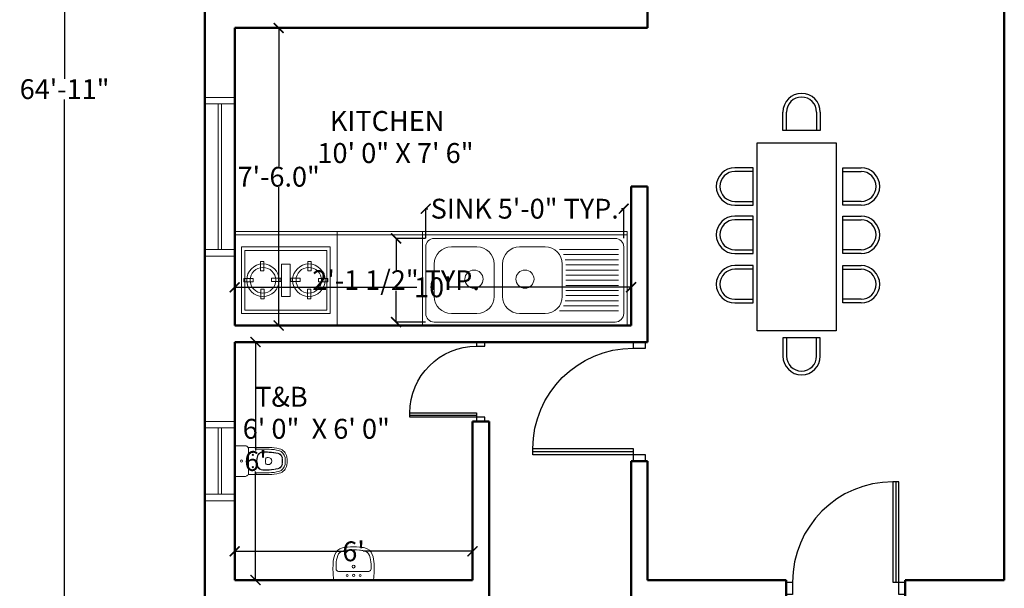
# Model space of a CAD drawing. Units: inches. Extents: x 147 to 1638, y 107 to 941.
# Tile 13 of 17: x 1062 to 1360, y 398 to 570. Entities that reach past the tile are written whole.
import ezdxf

# ---------------------------------------------------------------- set-up
doc = ezdxf.new("R2010")
doc.units = ezdxf.units.IN
doc.header["$MEASUREMENT"] = 0
for name, color, linetype, lineweight in [('A-ANNO-DIMS', 2, 'Continuous', 15), ('A-AREA-IDEN', 7, 'Continuous', 18), ('A-Door', 150, 'Continuous', 25), ('A-EQPM', 8, 'Continuous', 18), ('A-FLOR-CASE', 9, 'Continuous', 20), ('A-FLOR-FIXT', 9, 'Continuous', 18), ('furniture', 50, 'Continuous', 18), ('walls', 7, 'Continuous', 50), ('windows', 3, 'Continuous', 20)]:
    doc.layers.add(name, color=color, linetype=linetype, lineweight=lineweight)
for name, color, linetype in [('A-Glaz', 92, 'Continuous'), ('NT', 1, 'Continuous'), ('家', 40, 'Continuous')]:
    doc.layers.add(name, color=color, linetype=linetype)
doc.styles.get("Standard").update_dxf_attribs({"font": 'arial.ttf'})
doc.dimstyles.get("Standard").update_dxf_attribs({"dimtxt": 6, "dimasz": 3, "dimexe": 0.18, "dimexo": 0.0625, "dimgap": 0.09, "dimtad": 0, "dimtih": 1, "dimtoh": 1, "dimdec": 1, "dimzin": 0, "dimdsep": 46, "dimlunit": 3, "dimtxsty": 'Standard', "dimblk": 'ARCHTICK', "dimcen": 0.09, "dimadec": 0, "dimazin": 0, "dimtfac": 1, "dimtdec": 1, "dimtofl": 0, "dimtmove": 0, "dimatfit": 3, "dimfxl": 1, "dimtolj": 1, "dimtzin": 0, "dimarcsym": 0})

# ---------------------------------------------------------------- blocks, each defined once
blk = doc.blocks.new('A$C087A3AA9')
at = {"layer": 'A-Door'}
for points in [[(852.6, 94.7), (852.6, 852.6), (805.3, 852.6), (805.3, 94.7)], [(47.4, 94.7), (47.4, 0), (0, 0), (0, 94.7)], [(900, 94.7), (900, 0), (852.6, 0), (852.6, 94.7)]]:
    blk.add_lwpolyline(points, close=True, dxfattribs=at)
at = {"layer": 'A-Glaz'}
blk.add_line((828.9, 852.6), (828.9, 94.7), dxfattribs=at)
at = {"layer": 'NT'}
blk.add_arc((805.3, 94.7), 757.9, 90, 180, dxfattribs=at)
blk = doc.blocks.new('_ArchTick')
at = {"color": 0, "linetype": 'ByBlock', "const_width": 0.15}
blk.add_lwpolyline([(-0.5, -0.5), (0.5, 0.5)], dxfattribs=at)
blk = doc.blocks.new('*D59')
at = {"layer": 'A-ANNO-DIMS', "color": 0, "lineweight": -2, "transparency": 16777216}
for p, q in [((1133.05, 567.72), (1140.27, 567.72)), ((1140.09, 567.72), (1140.09, 525.87)), ((1140.09, 477.72), (1140.09, 519.56)), ((1133.05, 477.72), (1140.27, 477.72))]:
    blk.add_line(p, q, dxfattribs=at)
at = {"layer": 'Defpoints', "color": 0, "lineweight": -2, "transparency": 16777216}
for p in [(1132.98, 567.72), (1132.98, 477.72), (1140.09, 477.72)]:
    blk.add_point(p, dxfattribs=at)
at = {"layer": 'A-ANNO-DIMS', "color": 0, "lineweight": -2, "transparency": 16777216, "xscale": 3, "yscale": 3, "zscale": 3}
for p, rotation in [((1140.09, 567.72), 90), ((1140.09, 477.72), 270)]:
    blk.add_blockref('_ArchTick', p, dxfattribs=dict(at, rotation=rotation))
at = {"layer": 'A-ANNO-DIMS', "color": 0, "transparency": 16777216, "insert": (1140.09, 522.72), "char_height": 6, "attachment_point": 5}
blk.add_mtext('\\A1;7\'-6.0"', dxfattribs=at)
blk = doc.blocks.new('*D60')
at = {"layer": 'A-ANNO-DIMS', "color": 0, "lineweight": -2, "transparency": 16777216}
for p, q in [((1126.77, 486.05), (1126.77, 489.45)), ((1126.77, 489.27), (1181.87, 489.27)), ((1246.77, 489.27), (1191.67, 489.27)), ((1246.77, 486.05), (1246.77, 489.45))]:
    blk.add_line(p, q, dxfattribs=at)
at = {"layer": 'Defpoints', "color": 0, "lineweight": -2, "transparency": 16777216}
for p in [(1246.77, 489.27), (1126.77, 485.98), (1246.77, 485.98)]:
    blk.add_point(p, dxfattribs=at)
at = {"layer": 'A-ANNO-DIMS', "color": 0, "lineweight": -2, "transparency": 16777216, "xscale": 3, "yscale": 3, "zscale": 3, "rotation": 180}
blk.add_blockref('_ArchTick', (1126.77, 489.27), dxfattribs=at)
at = {"layer": 'A-ANNO-DIMS', "color": 0, "lineweight": -2, "transparency": 16777216, "xscale": 3, "yscale": 3, "zscale": 3}
blk.add_blockref('_ArchTick', (1246.77, 489.27), dxfattribs=at)
at = {"layer": 'A-ANNO-DIMS', "color": 0, "transparency": 16777216, "insert": (1186.77, 489.27), "char_height": 6, "attachment_point": 5}
blk.add_mtext("\\A1;10'", dxfattribs=at)
blk = doc.blocks.new('*D61')
at = {"layer": 'A-ANNO-DIMS', "color": 0, "lineweight": -2, "transparency": 16777216}
for p, q in [((1131.42, 472.72), (1133.26, 472.72)), ((1133.08, 472.72), (1133.08, 439.87)), ((1133.08, 400.72), (1133.08, 433.56)), ((1131.42, 400.72), (1133.26, 400.72))]:
    blk.add_line(p, q, dxfattribs=at)
at = {"layer": 'Defpoints', "color": 0, "lineweight": -2, "transparency": 16777216}
for p in [(1131.36, 472.72), (1131.36, 400.72), (1133.08, 400.72)]:
    blk.add_point(p, dxfattribs=at)
at = {"layer": 'A-ANNO-DIMS', "color": 0, "lineweight": -2, "transparency": 16777216, "xscale": 3, "yscale": 3, "zscale": 3}
for p, rotation in [((1133.08, 472.72), 90), ((1133.08, 400.72), 270)]:
    blk.add_blockref('_ArchTick', p, dxfattribs=dict(at, rotation=rotation))
at = {"layer": 'A-ANNO-DIMS', "color": 0, "transparency": 16777216, "insert": (1133.08, 436.72), "char_height": 6, "attachment_point": 5}
blk.add_mtext("\\A1;6'", dxfattribs=at)
blk = doc.blocks.new('*D62')
at = {"layer": 'A-ANNO-DIMS', "color": 0, "lineweight": -2, "transparency": 16777216}
for p, q in [((1126.77, 409.46), (1126.77, 409.58)), ((1126.77, 409.4), (1159.9, 409.4)), ((1198.77, 409.4), (1165.63, 409.4)), ((1198.77, 409.46), (1198.77, 409.58))]:
    blk.add_line(p, q, dxfattribs=at)
at = {"layer": 'Defpoints', "color": 0, "lineweight": -2, "transparency": 16777216}
for p in [(1126.77, 409.4), (1198.77, 409.4), (1198.77, 409.4)]:
    blk.add_point(p, dxfattribs=at)
at = {"layer": 'A-ANNO-DIMS', "color": 0, "lineweight": -2, "transparency": 16777216, "xscale": 3, "yscale": 3, "zscale": 3, "rotation": 180}
blk.add_blockref('_ArchTick', (1126.77, 409.4), dxfattribs=at)
at = {"layer": 'A-ANNO-DIMS', "color": 0, "lineweight": -2, "transparency": 16777216, "xscale": 3, "yscale": 3, "zscale": 3}
blk.add_blockref('_ArchTick', (1198.77, 409.4), dxfattribs=at)
at = {"layer": 'A-ANNO-DIMS', "color": 0, "transparency": 16777216, "insert": (1162.77, 409.4), "char_height": 6, "attachment_point": 5}
blk.add_mtext("\\A1;6'", dxfattribs=at)
blk = doc.blocks.new('2SAINDA')
at = {"color": 0, "linetype": 'ByBlock'}
for p, q in [((0, 0.188), (0, -0.188)), ((0.018, 0.2), (0.141, 0.2)), ((0.157, 0.192), (0.162, 0.188)), ((0.18, -0.164), (0.18, 0.164)), ((0.279, 0.159), (0.261, 0.176)), ((0.437, 0.047), (0.424, 0.047)), ((0.437, -0.047), (0.424, -0.047)), ((0.018, -0.2), (0.141, -0.2)), ((0.157, -0.192), (0.162, -0.188)), ((0.279, -0.159), (0.261, -0.176))]:
    blk.add_line(p, q, dxfattribs=at)
for centre, radius in [((0.09, 0), 0.0135), ((0.09, 0), 0.0135), ((0.236, 0.08), 0.0075), ((0.236, -0.08), 0.0075)]:
    blk.add_circle(centre, radius, dxfattribs=at)
for centre, radius, start, end in [((0.018, 0.18), 0.02, 90, 155.6901), ((0.141, 0.181), 0.019, 34.9372, 90), ((0.155, 0.164), 0.025, 23.3776, 73.7848), ((0.383, -5.322), 5.5, 89.2905, 92.1362), ((0.155, 0.164), 0.025, 360, 23.3776), ((0.293, 0.173), 0.02, 225, 270.9364), ((0.383, -5.322), 5.476, 89.2905, 90.9364), ((0.444, -0.373), 0.55, 75.4605, 89.2905), ((0.444, -0.373), 0.526, 75.4605, 89.2905), ((0.549, 0.03), 0.11, 8.8162, 75.4605), ((0.549, 0.03), 0.134, 8.8162, 75.4605), ((0.485, 0), 0.2, 160.016, 199.984), ((0.485, 0), 0.196, 160.016, 199.984), ((0.368, 0.043), 0.075, 90.1648, 160.016), ((0.368, 0.043), 0.071, 90.1648, 160.016), ((0.383, -5.322), 5.44, 89.2905, 90.1648), ((0.383, -5.322), 5.436, 89.2905, 90.1648), ((0.582, 0), 0.18, 170.2849, 189.7151), ((0.424, 0.027), 0.02, 90, 170.2849), ((0.437, 0), 0.047, 0, 90), ((0.437, 0), 0.047, 270, 0), ((0.444, -0.373), 0.49, 75.4605, 89.2905), ((0.444, -0.373), 0.486, 75.4605, 89.2905), ((0.549, 0.03), 0.07, 8.8162, 75.4605), ((0.549, 0.03), 0.074, 8.8162, 75.4605), ((0.355, 0), 0.266, 351.1838, 8.8162), ((0.355, 0), 0.27, 351.1838, 8.8162), ((0.355, 0), 0.306, 351.1838, 8.8162), ((0.355, 0), 0.33, 351.1838, 8.8162), ((0.368, -0.043), 0.075, 199.984, 269.8352), ((0.368, -0.043), 0.071, 199.984, 269.8352), ((0.383, 5.322), 5.436, 269.8352, 270.7095), ((0.383, 5.322), 5.44, 269.8352, 270.7095), ((0.424, -0.027), 0.02, 189.7151, 270), ((0.444, 0.373), 0.486, 270.7095, 284.5395), ((0.444, 0.373), 0.49, 270.7095, 284.5395), ((0.549, -0.03), 0.07, 284.5395, 351.1838), ((0.549, -0.03), 0.074, 284.5395, 351.1838), ((0.549, -0.03), 0.11, 284.5395, 351.1838), ((0.549, -0.03), 0.134, 284.5395, 351.1838), ((0.018, -0.18), 0.02, 204.3099, 270), ((0.141, -0.181), 0.019, 270, 325.0628), ((0.155, -0.164), 0.025, 286.2152, 336.6224), ((0.155, -0.164), 0.025, 336.6224, 0), ((0.383, 5.322), 5.5, 267.8638, 270.7095), ((0.293, -0.173), 0.02, 89.0636, 135), ((0.383, 5.322), 5.476, 269.0636, 270.7095), ((0.444, 0.373), 0.526, 270.7095, 284.5395), ((0.444, 0.373), 0.55, 270.7095, 284.5395)]:
    blk.add_arc(centre, radius, start, end, dxfattribs=at)
blk = doc.blocks.new('2SALADA2')
at = {"color": 0}
for p, q in [((-0.296, 0), (0.296, 0)), ((0.207, -0.13), (-0.207, -0.13))]:
    blk.add_line(p, q, dxfattribs=at)
for centre, radius in [((-0.1, -0.07), 0.015), ((0, -0.07), 0.0175), ((0.1, -0.07), 0.015), ((0, -0.205), 0.023)]:
    blk.add_circle(centre, radius, dxfattribs=at)
for centre, radius, start, end in [((-0.296, -0.01), 0.01, 90, 173.6262), ((0.296, -0.01), 0.01, 6.3738, 90), ((1.185, -0.175), 1.5, 173.6262, 182.693), ((-0.227, -0.171), 0.04, 95.5937, 179.6995), ((-0.207, -0.38), 0.25, 90, 95.5937), ((0.207, -0.38), 0.25, 84.4063, 90), ((0.227, -0.171), 0.04, 0.3005, 84.4063), ((-1.185, -0.175), 1.5, 357.307, 6.3738), ((0.186, -0.222), 0.5, 182.693, 199.3406), ((1.186, -0.221), 1.454, 178.0234, 180.898), ((0.186, -0.222), 0.454, 182.693, 199.3406), ((-0.186, -0.222), 0.454, 340.6594, 357.307), ((-1.186, -0.221), 1.454, 359.102, 1.9766), ((-0.186, -0.222), 0.5, 340.6594, 357.307), ((-0.135, -0.335), 0.16, 199.3406, 257.4429), ((-0.135, -0.335), 0.114, 199.3406, 257.4429), ((-0.061, -0.003), 0.454, 257.4429, 266.4982), ((0.061, -0.003), 0.454, 273.5018, 282.5571), ((0.135, -0.335), 0.114, 282.5571, 340.6594), ((0.135, -0.335), 0.16, 282.5571, 340.6594), ((-0.061, -0.003), 0.5, 257.4429, 266.4982), ((0, 0.995), 1.5, 266.4982, 273.5018), ((0, 0.995), 1.454, 266.4982, 273.5018), ((0.061, -0.003), 0.5, 273.5018, 282.5571)]:
    blk.add_arc(centre, radius, start, end, dxfattribs=at)
blk = doc.blocks.new('A$C45A766E2')
at = {"layer": '家'}
for p, q in [((0.363, 1.317), (0.363, 1.078)), ((0.412, 1.317), (0.412, 1.078)), ((0.801, 1.078), (0.801, 1.317)), ((0.849, 1.078), (0.849, 1.317)), ((1.006, 1.317), (1.006, 1.078)), ((1.054, 1.317), (1.054, 1.078)), ((1.443, 1.078), (1.443, 1.317)), ((1.492, 1.078), (1.492, 1.317)), ((1.634, 1.317), (1.634, 1.078)), ((1.683, 1.317), (1.683, 1.078)), ((2.072, 1.078), (2.072, 1.317)), ((2.12, 1.078), (2.12, 1.317)), ((0, 1.028), (2.445, 1.028)), ((0, 0), (0, 1.028)), ((0.363, 1.078), (0.849, 1.078)), ((0.363, 1.078), (0.849, 1.078)), ((1.006, 1.078), (1.492, 1.078)), ((1.006, 1.078), (1.492, 1.078)), ((1.634, 1.078), (2.12, 1.078)), ((1.634, 1.078), (2.12, 1.078)), ((2.445, 1.028), (2.445, 0)), ((-0.088, 0.693), (-0.327, 0.693)), ((-0.088, 0.644), (-0.327, 0.644)), ((-0.088, 0.207), (-0.088, 0.693)), ((-0.088, 0.207), (-0.088, 0.693)), ((2.604, 0.693), (2.843, 0.693)), ((2.604, 0.207), (2.604, 0.693)), ((2.604, 0.207), (2.604, 0.693)), ((2.604, 0.644), (2.843, 0.644)), ((-0.327, 0.255), (-0.088, 0.255)), ((-0.327, 0.207), (-0.088, 0.207)), ((2.843, 0.255), (2.604, 0.255)), ((2.843, 0.207), (2.604, 0.207)), ((2.445, 0), (0, 0)), ((0.363, -0.085), (0.849, -0.085)), ((0.363, -0.085), (0.849, -0.085)), ((0.363, -0.324), (0.363, -0.085)), ((0.412, -0.324), (0.412, -0.085)), ((0.801, -0.085), (0.801, -0.324)), ((0.849, -0.085), (0.849, -0.324)), ((1.006, -0.324), (1.006, -0.085)), ((1.006, -0.085), (1.492, -0.085)), ((1.006, -0.085), (1.492, -0.085)), ((1.054, -0.324), (1.054, -0.085)), ((1.443, -0.085), (1.443, -0.324)), ((1.492, -0.085), (1.492, -0.324)), ((1.634, -0.085), (2.12, -0.085)), ((1.634, -0.085), (2.12, -0.085)), ((1.634, -0.324), (1.634, -0.085)), ((1.683, -0.324), (1.683, -0.085)), ((2.072, -0.085), (2.072, -0.324)), ((2.12, -0.085), (2.12, -0.324))]:
    blk.add_line(p, q, dxfattribs=at)
for centre, radius, start, end in [((0.606, 1.317), 0.243, 0, 180), ((1.249, 1.317), 0.243, 0, 180), ((1.877, 1.317), 0.243, 0, 180), ((0.606, 1.317), 0.195, 0, 180), ((1.249, 1.317), 0.195, 0, 180), ((1.877, 1.317), 0.195, 0, 180), ((-0.327, 0.45), 0.243, 90, 270), ((-0.327, 0.45), 0.195, 90, 270), ((2.843, 0.45), 0.243, 270, 90), ((2.843, 0.45), 0.195, 270, 90), ((0.606, -0.324), 0.243, 180, 0), ((0.606, -0.324), 0.195, 180, 0), ((1.249, -0.324), 0.243, 180, 0), ((1.249, -0.324), 0.195, 180, 0), ((1.877, -0.324), 0.243, 180, 0), ((1.877, -0.324), 0.195, 180, 0)]:
    blk.add_arc(centre, radius, start, end, dxfattribs=at)
blk = doc.blocks.new('WIN-48IN')
for p, q in [((9, 48), (0, 48)), ((0, 48), (0, 0)), ((9, 0), (9, 48)), ((9, 46), (0, 46)), ((4, 2), (4, 46)), ((5, 2), (5, 46)), ((0, 2), (9, 2)), ((0, 0), (9, 0))]:
    blk.add_line(p, q)
blk = doc.blocks.new('WIN-24IN')
for p, q in [((9, 24), (0, 24)), ((0, 24), (0, 0)), ((9, 0), (9, 24)), ((9, 22), (0, 22)), ((4, 2), (4, 22)), ((5, 2), (5, 22)), ((0, 2), (9, 2)), ((0, 0), (9, 0))]:
    blk.add_line(p, q)
blk = doc.blocks.new('CABINET-KITCHEN-RUN')
for p, q in [((0, 28.41), (118.8, 28.41)), ((0, 0), (0, 28.41)), ((0, 27.38), (118.8, 27.38)), ((30.99, 0), (30.99, 28.41)), ((56.82, 0), (56.82, 28.41)), ((118.8, 28.41), (118.8, 0)), ((118.8, 0), (0, 0))]:
    blk.add_line(p, q)
blk = doc.blocks.new('COOKTOP-2-BURNER')
for p, q in [((0, 0), (0, 20.15)), ((0, 20.15), (26.86, 20.15)), ((1.03, 1.03), (1.03, 19.11)), ((1.03, 19.11), (25.83, 19.11)), ((25.83, 1.03), (25.83, 19.11)), ((26.86, 0), (26.86, 20.15)), ((5.75, 15.75), (5.75, 12.91)), ((5.75, 15.75), (6.79, 15.75)), ((6.79, 15.75), (6.79, 12.91)), ((12.14, 14.98), (14.72, 14.98)), ((12.14, 14.98), (12.14, 5.17)), ((14.72, 14.98), (14.72, 5.17)), ((21.11, 15.75), (20.07, 15.75)), ((20.07, 15.75), (20.07, 12.91)), ((21.11, 15.75), (21.11, 12.91)), ((5.75, 12.91), (6.79, 12.91)), ((21.11, 12.91), (20.07, 12.91)), ((0.69, 9.55), (0.69, 10.59)), ((0.69, 10.59), (3.53, 10.59)), ((0.69, 9.55), (3.53, 9.55)), ((3.53, 9.55), (3.53, 10.59)), ((11.95, 10.69), (9.11, 10.69)), ((9.11, 10.69), (9.11, 9.66)), ((11.95, 9.66), (9.11, 9.66)), ((11.95, 10.69), (11.95, 9.66)), ((14.91, 10.69), (17.75, 10.69)), ((14.91, 10.69), (14.91, 9.66)), ((14.91, 9.66), (17.75, 9.66)), ((17.75, 10.69), (17.75, 9.66)), ((23.33, 9.55), (23.33, 10.59)), ((26.17, 10.59), (23.33, 10.59)), ((26.17, 9.55), (23.33, 9.55)), ((26.17, 9.55), (26.17, 10.59)), ((5.86, 4.49), (5.86, 7.33)), ((6.89, 7.33), (5.86, 7.33)), ((6.89, 4.49), (6.89, 7.33)), ((19.97, 4.49), (19.97, 7.33)), ((19.97, 7.33), (21, 7.33)), ((21, 4.49), (21, 7.33)), ((6.89, 4.49), (5.86, 4.49)), ((12.14, 5.17), (14.72, 5.17)), ((19.97, 4.49), (21, 4.49)), ((0, 0), (26.86, 0)), ((1.03, 1.03), (25.83, 1.03))]:
    blk.add_line(p, q)
for centre, radius in [((6.48, 10.08), 4.91), ((20.38, 10.08), 4.91), ((6.48, 10.08), 3.87), ((20.38, 10.08), 3.87)]:
    blk.add_circle(centre, radius)
blk = doc.blocks.new('SINK-DOUBLE-DRAINBOARD')
for p, q in [((57.34, 25.31), (2.58, 25.31)), ((0, 22.73), (0, 2.58)), ((15.5, 22.73), (7.75, 22.73)), ((36.16, 22.73), (28.41, 22.73)), ((40.53, 21.95), (58.37, 21.95)), ((59.92, 2.58), (59.92, 22.73)), ((41.67, 20.4), (58.37, 20.4)), ((42.22, 18.85), (58.37, 18.85)), ((2.58, 17.56), (2.58, 7.75)), ((20.66, 17.56), (20.66, 7.75)), ((23.24, 17.56), (23.24, 7.75)), ((41.32, 17.56), (41.32, 7.75)), ((42.36, 17.3), (58.37, 17.3)), ((42.36, 15.75), (58.37, 15.75)), ((42.36, 14.2), (58.37, 14.2)), ((42.36, 12.66), (58.37, 12.66)), ((42.36, 11.11), (58.37, 11.11)), ((42.36, 9.56), (58.37, 9.56)), ((42.22, 6.46), (58.37, 6.46)), ((42.36, 8.01), (58.37, 8.01)), ((40.53, 3.36), (58.37, 3.36)), ((41.67, 4.91), (58.37, 4.91)), ((2.58, 0), (57.34, 0)), ((7.75, 2.58), (15.5, 2.58)), ((28.41, 2.58), (36.16, 2.58))]:
    blk.add_line(p, q)
for centre in [(14.61, 13), (30.02, 13)]:
    blk.add_circle(centre, 2.75)
for centre, radius, start, end in [((2.58, 22.73), 2.58, 90, 180), ((57.34, 22.73), 2.58, 0, 90), ((7.75, 17.56), 5.17, 90, 180), ((15.5, 17.56), 5.17, 0, 90), ((28.41, 17.56), 5.17, 90, 180), ((36.16, 17.56), 5.17, 0, 90), ((7.75, 7.75), 5.17, 180, 270), ((15.5, 7.75), 5.17, 270, 0), ((28.41, 7.75), 5.17, 180, 270), ((36.16, 7.75), 5.17, 270, 0), ((2.58, 2.58), 2.58, 180, 270), ((57.34, 2.58), 2.58, 270, 0)]:
    blk.add_arc(centre, radius, start, end)
blk = doc.blocks.new('*D126')
at = {"layer": 'A-ANNO-DIMS', "color": 0, "lineweight": -2, "transparency": 16777216}
for p, q in [((1184.62, 504.12), (1184.62, 513.23)), ((1184.62, 513.05), (1185.27, 513.05)), ((1244.54, 513.05), (1243.89, 513.05)), ((1244.54, 504.12), (1244.54, 513.23))]:
    blk.add_line(p, q, dxfattribs=at)
at = {"layer": 'Defpoints', "color": 0, "lineweight": -2, "transparency": 16777216}
for p in [(1244.54, 513.05), (1184.62, 504.06), (1244.54, 504.06)]:
    blk.add_point(p, dxfattribs=at)
at = {"layer": 'A-ANNO-DIMS', "color": 0, "lineweight": -2, "transparency": 16777216, "xscale": 3, "yscale": 3, "zscale": 3, "rotation": 180}
blk.add_blockref('_ArchTick', (1184.62, 513.05), dxfattribs=at)
at = {"layer": 'A-ANNO-DIMS', "color": 0, "lineweight": -2, "transparency": 16777216, "xscale": 3, "yscale": 3, "zscale": 3}
blk.add_blockref('_ArchTick', (1244.54, 513.05), dxfattribs=at)
at = {"layer": 'A-ANNO-DIMS', "color": 0, "transparency": 16777216, "insert": (1214.58, 513.05), "char_height": 6, "attachment_point": 5}
blk.add_mtext('\\A1;SINK 5\'-0" TYP.', dxfattribs=at)
blk = doc.blocks.new('*D127')
at = {"layer": 'A-ANNO-DIMS', "color": 0, "lineweight": -2, "transparency": 16777216}
for p, q in [((1184.56, 504.06), (1175.45, 504.06)), ((1175.63, 504.06), (1175.63, 494.6)), ((1175.63, 478.75), (1175.63, 488.21)), ((1184.56, 478.75), (1175.45, 478.75))]:
    blk.add_line(p, q, dxfattribs=at)
at = {"layer": 'Defpoints', "color": 0, "lineweight": -2, "transparency": 16777216}
for p in [(1175.63, 504.06), (1184.62, 504.06), (1184.62, 478.75)]:
    blk.add_point(p, dxfattribs=at)
at = {"layer": 'A-ANNO-DIMS', "color": 0, "lineweight": -2, "transparency": 16777216, "xscale": 3, "yscale": 3, "zscale": 3}
for p, rotation in [((1175.63, 504.06), 90), ((1175.63, 478.75), 270)]:
    blk.add_blockref('_ArchTick', p, dxfattribs=dict(at, rotation=rotation))
at = {"layer": 'A-ANNO-DIMS', "color": 0, "transparency": 16777216, "insert": (1175.63, 491.41), "char_height": 6, "attachment_point": 5}
blk.add_mtext('\\A1;2\'-1 1/2" TYP.', dxfattribs=at)
blk = doc.blocks.new('*D135')
at = {"layer": 'A-ANNO-DIMS', "color": 0, "lineweight": -2, "transparency": 16777216}
for p, q in [((1176.71, 938.72), (1075.09, 938.72)), ((1075.27, 938.72), (1075.27, 552.37)), ((1075.27, 159.72), (1075.27, 546.06)), ((1117.71, 159.72), (1075.09, 159.72))]:
    blk.add_line(p, q, dxfattribs=at)
at = {"layer": 'Defpoints', "color": 0, "lineweight": -2, "transparency": 16777216}
for p in [(1075.27, 938.72), (1176.77, 938.72), (1117.77, 159.72)]:
    blk.add_point(p, dxfattribs=at)
at = {"layer": 'A-ANNO-DIMS', "color": 0, "lineweight": -2, "transparency": 16777216, "xscale": 3, "yscale": 3, "zscale": 3}
for p, rotation in [((1075.27, 938.72), 90), ((1075.27, 159.72), 270)]:
    blk.add_blockref('_ArchTick', p, dxfattribs=dict(at, rotation=rotation))
at = {"layer": 'A-ANNO-DIMS', "color": 0, "transparency": 16777216, "insert": (1075.27, 549.22), "char_height": 6, "attachment_point": 5}
blk.add_mtext('\\A1;64\'-11"', dxfattribs=at)

msp = doc.modelspace()

# ---------------------------------------------------------------- linework, layer by layer
at = {"layer": 'walls'}
for p, q in [((1117.77, 909.72), (1117.77, 201.72)), ((1359.77, 722.72), (1359.77, 400.72)), ((1251.77, 572.72), (1251.77, 567.72)), ((1126.77, 567.72), (1126.77, 477.72)), ((1126.77, 567.72), (1246.77, 567.72)), ((1246.77, 567.72), (1251.77, 567.72)), ((1246.77, 519.72), (1246.77, 477.72)), ((1246.77, 519.72), (1251.77, 519.72)), ((1251.77, 519.72), (1251.77, 472.72)), ((1126.77, 477.72), (1246.77, 477.72)), ((1126.77, 472.72), (1126.77, 400.72)), ((1126.77, 472.72), (1198.77, 472.72)), ((1203.77, 472.72), (1198.77, 472.72)), ((1203.77, 472.72), (1246.77, 472.72)), ((1246.77, 472.72), (1251.77, 472.72)), ((1198.77, 448.72), (1198.77, 400.72)), ((1203.77, 448.72), (1198.77, 448.72)), ((1203.77, 448.72), (1203.77, 395.72)), ((1246.77, 436.72), (1246.77, 210.72)), ((1246.77, 436.72), (1251.77, 436.72)), ((1251.77, 436.72), (1251.77, 400.72)), ((1126.77, 400.72), (1198.77, 400.72)), ((1251.77, 400.72), (1281.77, 400.72)), ((1281.77, 400.72), (1293.77, 400.72)), ((1293.77, 400.72), (1293.77, 395.72)), ((1329.77, 400.72), (1359.77, 400.72)), ((1329.77, 400.72), (1329.77, 395.72))]:
    msp.add_line(p, q, dxfattribs=at)

# ---------------------------------------------------------------- block references
at = {"layer": 'A-Door', "rotation": 90}
for p, xscale, yscale, zscale in [((1202.53, 472.72), -0.0266666667542921, 0.0266666667542921, 0.0266666667542921), ((1251.16, 472.72), -0.0400000000000001, 0.0400000000000001, 0.0400000000000001)]:
    msp.add_blockref('A$C087A3AA9', p, dxfattribs=dict(at, xscale=xscale, yscale=yscale, zscale=zscale))
at = {"layer": 'A-Door', "xscale": 0.0400000000000001, "yscale": 0.0400000000000001, "zscale": 0.0400000000000001}
msp.add_blockref('A$C087A3AA9', (1293.77, 396.32), dxfattribs=at)
at = {"layer": 'A-EQPM'}
msp.add_blockref('COOKTOP-2-BURNER', (1128.83, 481.33), dxfattribs=at)
at = {"layer": 'A-FLOR-CASE'}
msp.add_blockref('CABINET-KITCHEN-RUN', (1126.77, 477.72), dxfattribs=at)
at = {"layer": 'A-FLOR-FIXT'}
msp.add_blockref('SINK-DOUBLE-DRAINBOARD', (1184.62, 478.75), dxfattribs=at)
at = {"layer": 'A-FLOR-FIXT', "xscale": 23.19012112898009, "yscale": 23.19012112898009, "zscale": 23.19012112898009}
msp.add_blockref('2SAINDA', (1126.77, 436.72), dxfattribs=at)
at = {"layer": 'A-FLOR-FIXT', "xscale": 19.81841434140962, "yscale": 19.81841434140962, "zscale": 19.81841434140962, "rotation": 180}
msp.add_blockref('2SALADA2', (1162.77, 400.72), dxfattribs=at)
at = {"layer": 'furniture', "xscale": 23.28367368005433, "yscale": 23.28367368005433, "zscale": 23.28367368005433, "rotation": 90}
msp.add_blockref('A$C45A766E2', (1308.87, 476.07), dxfattribs=at)
at = {"layer": 'windows'}
for name, p in [('WIN-48IN', (1117.77, 498.72)), ('WIN-24IN', (1117.77, 424.72))]:
    msp.add_blockref(name, p, dxfattribs=at)

# ---------------------------------------------------------------- texts
at = {"layer": 'A-AREA-IDEN'}
for s, height, p in [('KITCHEN ', 6.031, (1155.57, 536.56)), ('  10\' 0" X 7\' 6"', 6.0306, (1148.12, 526.87)), ('T&B', 6.031, (1132.95, 453.14)), ('  6\' 0"  X 6\' 0"', 6.0306, (1125.51, 443.45))]:
    msp.add_text(s, height=height, dxfattribs=at).set_placement(p)

# ---------------------------------------------------------------- dimensions: what is measured, and where the dimension line sits
at = {"layer": 'A-ANNO-DIMS'}
for base, p1, p2, override, picture, middle in [((1075.27, 938.72), (1117.77, 159.72), (1176.77, 938.72), {"dimdec": 1, "dimlfac": 1, "dimrnd": 0, "dimzin": 1, "dimdsep": 46, "dimlunit": 4, "dimfrac": 2}, '*D135', (1075.27, 549.22)), ((1140.09, 477.72), (1132.98, 567.72), (1132.98, 477.72), {"dimclrd": 0, "dimclre": 0, "dimclrt": 0}, '*D59', (1140.09, 522.72)), ((1133.08, 400.72), (1131.36, 472.72), (1131.36, 400.72), {"dimclrd": 0, "dimclre": 0, "dimclrt": 0}, '*D61', (1133.08, 436.72))]:
    dim = msp.add_linear_dim(base=base, p1=p1, p2=p2, angle=90, dimstyle='Standard', override=override, dxfattribs=at)
    dim.commit()
    dim.dimension.update_dxf_attribs({"geometry": picture, "text_midpoint": middle})
dim = msp.add_linear_dim(base=(1244.54, 513.05), p1=(1184.62, 504.06), p2=(1244.54, 504.06), text='SINK <> TYP.', dimstyle='Standard', override={"dimdec": 1, "dimlfac": 1, "dimrnd": 0, "dimzin": 1, "dimdsep": 46, "dimlunit": 4, "dimfrac": 2}, dxfattribs=at)
dim.commit()
dim.dimension.update_dxf_attribs({"geometry": '*D126', "text_midpoint": (1214.58, 513.05)})
dim = msp.add_linear_dim(base=(1175.63, 504.06), p1=(1184.62, 478.75), p2=(1184.62, 504.06), angle=90, text='<> TYP.', dimstyle='Standard', override={"dimdec": 1, "dimlfac": 1, "dimrnd": 0, "dimzin": 1, "dimdsep": 46, "dimlunit": 4, "dimfrac": 2}, dxfattribs=at)
dim.commit()
dim.dimension.update_dxf_attribs({"geometry": '*D127', "text_midpoint": (1175.63, 491.41)})
for base, p1, p2, picture, middle in [((1246.77, 489.27), (1126.77, 485.98), (1246.77, 485.98), '*D60', (1186.77, 489.27)), ((1198.77, 409.4), (1126.77, 409.4), (1198.77, 409.4), '*D62', (1162.77, 409.4))]:
    dim = msp.add_linear_dim(base=base, p1=p1, p2=p2, dimstyle='Standard', override={"dimclrd": 0, "dimclre": 0, "dimclrt": 0}, dxfattribs=at)
    dim.commit()
    dim.dimension.update_dxf_attribs({"geometry": picture, "text_midpoint": middle})

doc.saveas('drawing.dxf')
